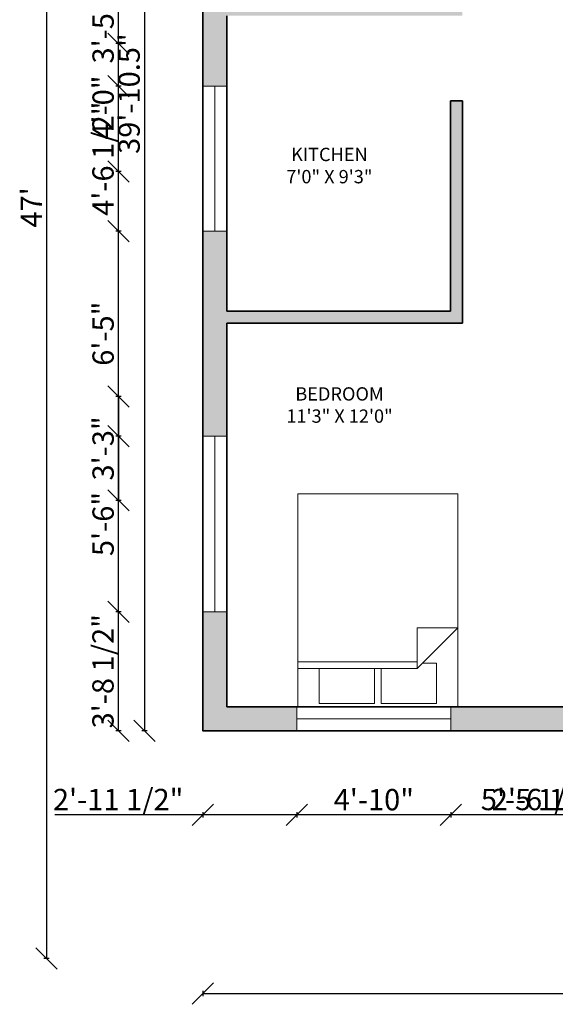
# Model space of a CAD drawing. Units: inches. Extents: x 2561 to 3163, y 493 to 1211.
# Tile 1 of 8: x 2561 to 2762, y 512 to 882. Entities that reach past the tile are written whole.
import ezdxf

# ---------------------------------------------------------------- set-up
doc = ezdxf.new("R2010")
doc.units = ezdxf.units.IN
for name, color, linetype, lineweight in [('A-ANNO-DIMS', 2, 'Continuous', 18), ('A-AREA-IDEN', 7, 'Continuous', 18), ('A-FURN', 8, 'Continuous', 18), ('A-GLAZ', 4, 'Continuous', 18), ('A-WALL', 7, 'Continuous', 35), ('A-WALL-PATT', 24, 'Continuous', 13)]:
    doc.layers.add(name, color=color, linetype=linetype, lineweight=lineweight)
doc.styles.get("Standard").update_dxf_attribs({"font": 'arial.ttf'})
doc.dimstyles.new('ISO-25', dxfattribs={"dimtxt": 8, "dimasz": 8, "dimexe": 1, "dimexo": 1, "dimtad": 1, "dimlunit": 3, "dimtxsty": 'Standard', "dimblk": 'OBLIQUE', "dimcen": 2.5, "dimadec": 0, "dimazin": 0, "dimtfac": 1, "dimtmove": 0, "dimatfit": 3, "dimfxl": 1, "dimfxlon": 1, "dimarcsym": 0})

# ---------------------------------------------------------------- blocks, each defined once
blk = doc.blocks.new('Bed - Queen')
for p, q in [((0, -80.00003), (0, 0)), ((0, 0), (59.99999, 0)), ((59.99999, 0), (59.99999, -80.00003)), ((7.99999, -1.2), (28.79998, -1.2)), ((7.99999, -14.4), (7.99999, -1.2)), ((28.79998, -1.2), (28.79998, -14.4)), ((31.19999, -1.2), (51.99999, -1.2)), ((31.19999, -14.4), (31.19999, -1.2)), ((51.99999, -1.2), (51.99999, -16.4)), ((0, -14.4), (44.8, -14.4)), ((59.99999, -29.6), (44.8, -14.4)), ((44.8, -14.4), (44.8, -29.6)), ((44.8, -16.8), (0, -16.8)), ((51.99999, -16.4), (46.79936, -16.4)), ((44.8, -29.6), (59.99999, -29.6)), ((59.99999, -80.00003), (0, -80.00003))]:
    blk.add_line(p, q)
blk = doc.blocks.new('_Oblique')
at = {"color": 0, "linetype": 'ByBlock', "lineweight": -2}
blk.add_line((-0.5, -0.5), (0.5, 0.5), dxfattribs=at)
blk = doc.blocks.new('*D15')
at = {"layer": 'A-ANNO-DIMS', "color": 0, "lineweight": -2, "transparency": 16777216}
for p, q in [((2629.27, 516.82), (2629.27, 514.82)), ((2629.27, 515.82), (2948.92, 515.82)), ((2948.92, 516.82), (2948.92, 514.82))]:
    blk.add_line(p, q, dxfattribs=at)
at = {"layer": 'Defpoints', "color": 0, "transparency": 16777216}
for p in [(2629.27, 614.57), (2948.92, 614.57), (2948.92, 515.82)]:
    blk.add_point(p, dxfattribs=at)
at = {"layer": 'A-ANNO-DIMS', "color": 0, "lineweight": -2, "transparency": 16777216, "xscale": 8, "yscale": 8, "zscale": 8, "rotation": 180}
blk.add_blockref('_Oblique', (2629.27, 515.82), dxfattribs=at)
at = {"layer": 'A-ANNO-DIMS', "color": 0, "lineweight": -2, "transparency": 16777216, "xscale": 8, "yscale": 8, "zscale": 8}
blk.add_blockref('_Oblique', (2948.92, 515.82), dxfattribs=at)
at = {"layer": 'A-ANNO-DIMS', "color": 0, "transparency": 16777216, "insert": (2789.1, 520.53), "char_height": 8, "attachment_point": 5}
blk.add_mtext('26\'-7.64"', dxfattribs=at)
blk = doc.blocks.new('*D16')
at = {"layer": 'A-ANNO-DIMS', "color": 0, "lineweight": -2, "transparency": 16777216}
for p, q in [((2608.39, 1093.07), (2606.39, 1093.07)), ((2607.39, 1093.07), (2607.39, 614.57)), ((2608.39, 614.57), (2606.39, 614.57))]:
    blk.add_line(p, q, dxfattribs=at)
at = {"layer": 'Defpoints', "color": 0, "transparency": 16777216}
for p in [(2629.27, 1093.07), (2607.39, 614.57), (2629.27, 614.57)]:
    blk.add_point(p, dxfattribs=at)
at = {"layer": 'A-ANNO-DIMS', "color": 0, "lineweight": -2, "transparency": 16777216, "xscale": 8, "yscale": 8, "zscale": 8}
for p, rotation in [((2607.39, 1093.07), 90), ((2607.39, 614.57), 270)]:
    blk.add_blockref('_Oblique', p, dxfattribs=dict(at, rotation=rotation))
at = {"layer": 'A-ANNO-DIMS', "color": 0, "transparency": 16777216, "insert": (2602.67, 853.82), "char_height": 8, "attachment_point": 5, "rotation": 90}
blk.add_mtext('39\'-10.5"', dxfattribs=at)
blk = doc.blocks.new('*D17')
at = {"layer": 'A-ANNO-DIMS', "color": 0, "lineweight": -2, "transparency": 16777216}
for p, q in [((2571.63, 1093.07), (2569.63, 1093.07)), ((2570.63, 1093.07), (2570.63, 529.07)), ((2571.63, 529.07), (2569.63, 529.07))]:
    blk.add_line(p, q, dxfattribs=at)
at = {"layer": 'Defpoints', "color": 0, "transparency": 16777216}
for p in [(2629.27, 1093.07), (2570.63, 529.07), (3109.27, 529.07)]:
    blk.add_point(p, dxfattribs=at)
at = {"layer": 'A-ANNO-DIMS', "color": 0, "lineweight": -2, "transparency": 16777216, "xscale": 8, "yscale": 8, "zscale": 8}
for p, rotation in [((2570.63, 1093.07), 90), ((2570.63, 529.07), 270)]:
    blk.add_blockref('_Oblique', p, dxfattribs=dict(at, rotation=rotation))
at = {"layer": 'A-ANNO-DIMS', "color": 0, "transparency": 16777216, "insert": (2566, 811.07), "char_height": 8, "attachment_point": 5, "rotation": 90}
blk.add_mtext("47'", dxfattribs=at)
blk = doc.blocks.new('*D30')
at = {"layer": 'A-ANNO-DIMS', "color": 0, "lineweight": -2, "transparency": 16777216}
for p, q in [((2598.62, 740.07), (2596.62, 740.07)), ((2597.62, 740.07), (2597.62, 701.07)), ((2598.62, 701.07), (2596.62, 701.07))]:
    blk.add_line(p, q, dxfattribs=at)
at = {"layer": 'Defpoints', "color": 0, "transparency": 16777216}
for p in [(3014.77, 740.07), (2597.62, 701.07), (3014.77, 701.07)]:
    blk.add_point(p, dxfattribs=at)
at = {"layer": 'A-ANNO-DIMS', "color": 0, "lineweight": -2, "transparency": 16777216, "xscale": 8, "yscale": 8, "zscale": 8}
for p, rotation in [((2597.62, 740.07), 90), ((2597.62, 701.07), 270)]:
    blk.add_blockref('_Oblique', p, dxfattribs=dict(at, rotation=rotation))
at = {"layer": 'A-ANNO-DIMS', "color": 0, "transparency": 16777216, "insert": (2592.91, 720.57), "char_height": 8, "attachment_point": 5, "rotation": 90}
blk.add_mtext('3\'-3"', dxfattribs=at)
blk = doc.blocks.new('*D31')
at = {"layer": 'A-ANNO-DIMS', "color": 0, "lineweight": -2, "transparency": 16777216}
for p, q in [((2598.62, 872.57), (2596.62, 872.57)), ((2597.62, 824.57), (2597.62, 872.57)), ((2598.62, 824.57), (2596.62, 824.57))]:
    blk.add_line(p, q, dxfattribs=at)
at = {"layer": 'Defpoints', "color": 0, "transparency": 16777216}
for p in [(2597.62, 872.57), (3011.27, 872.57), (3011.27, 824.57)]:
    blk.add_point(p, dxfattribs=at)
at = {"layer": 'A-ANNO-DIMS', "color": 0, "lineweight": -2, "transparency": 16777216, "xscale": 8, "yscale": 8, "zscale": 8}
for p, rotation in [((2597.62, 872.57), 90), ((2597.62, 824.57), 270)]:
    blk.add_blockref('_Oblique', p, dxfattribs=dict(at, rotation=rotation))
at = {"layer": 'A-ANNO-DIMS', "color": 0, "transparency": 16777216, "insert": (2592.91, 848.57), "char_height": 8, "attachment_point": 5, "rotation": 90}
blk.add_mtext('4\'-0"', dxfattribs=at)
blk = doc.blocks.new('*D46')
at = {"layer": 'A-ANNO-DIMS', "color": 0, "lineweight": -2, "transparency": 16777216}
for p, q in [((2598.62, 897.75), (2596.62, 897.75)), ((2597.62, 856.59), (2597.62, 897.75)), ((2598.62, 856.59), (2596.62, 856.59))]:
    blk.add_line(p, q, dxfattribs=at)
at = {"layer": 'Defpoints', "color": 0, "transparency": 16777216}
for p in [(2597.62, 897.75), (2629.27, 897.75), (2629.27, 856.59)]:
    blk.add_point(p, dxfattribs=at)
at = {"layer": 'A-ANNO-DIMS', "color": 0, "lineweight": -2, "transparency": 16777216, "xscale": 8, "yscale": 8, "zscale": 8}
for p, rotation in [((2597.62, 897.75), 90), ((2597.62, 856.59), 270)]:
    blk.add_blockref('_Oblique', p, dxfattribs=dict(at, rotation=rotation))
at = {"layer": 'A-ANNO-DIMS', "color": 0, "transparency": 16777216, "insert": (2592.91, 877.17), "char_height": 8, "attachment_point": 5, "rotation": 90}
blk.add_mtext('3\'-5"', dxfattribs=at)
blk = doc.blocks.new('*D47')
at = {"layer": 'A-ANNO-DIMS', "color": 0, "lineweight": -2, "transparency": 16777216}
for p, q in [((2598.62, 856.59), (2596.62, 856.59)), ((2597.62, 802.18), (2597.62, 856.59)), ((2598.62, 802.18), (2596.62, 802.18))]:
    blk.add_line(p, q, dxfattribs=at)
at = {"layer": 'Defpoints', "color": 0, "transparency": 16777216}
for p in [(2597.62, 856.59), (2629.27, 856.59), (2629.27, 802.18)]:
    blk.add_point(p, dxfattribs=at)
at = {"layer": 'A-ANNO-DIMS', "color": 0, "lineweight": -2, "transparency": 16777216, "xscale": 8, "yscale": 8, "zscale": 8}
for p, rotation in [((2597.62, 856.59), 90), ((2597.62, 802.18), 270)]:
    blk.add_blockref('_Oblique', p, dxfattribs=dict(at, rotation=rotation))
at = {"layer": 'A-ANNO-DIMS', "color": 0, "transparency": 16777216, "insert": (2592.86, 829.38), "char_height": 8, "attachment_point": 5, "rotation": 90}
blk.add_mtext('4\'-6 1/2"', dxfattribs=at)
blk = doc.blocks.new('*D48')
at = {"layer": 'A-ANNO-DIMS', "color": 0, "lineweight": -2, "transparency": 16777216}
for p, q in [((2598.62, 802.18), (2596.62, 802.18)), ((2597.62, 725.14), (2597.62, 802.18)), ((2598.62, 725.14), (2596.62, 725.14))]:
    blk.add_line(p, q, dxfattribs=at)
at = {"layer": 'Defpoints', "color": 0, "transparency": 16777216}
for p in [(2597.62, 802.18), (2629.27, 802.18), (2629.27, 725.14)]:
    blk.add_point(p, dxfattribs=at)
at = {"layer": 'A-ANNO-DIMS', "color": 0, "lineweight": -2, "transparency": 16777216, "xscale": 8, "yscale": 8, "zscale": 8}
for p, rotation in [((2597.62, 802.18), 90), ((2597.62, 725.14), 270)]:
    blk.add_blockref('_Oblique', p, dxfattribs=dict(at, rotation=rotation))
at = {"layer": 'A-ANNO-DIMS', "color": 0, "transparency": 16777216, "insert": (2592.91, 763.66), "char_height": 8, "attachment_point": 5, "rotation": 90}
blk.add_mtext('6\'-5"', dxfattribs=at)
blk = doc.blocks.new('*D49')
at = {"layer": 'A-ANNO-DIMS', "color": 0, "lineweight": -2, "transparency": 16777216}
for p, q in [((2598.62, 725.14), (2596.62, 725.14)), ((2597.62, 659.23), (2597.62, 725.14)), ((2598.62, 659.23), (2596.62, 659.23))]:
    blk.add_line(p, q, dxfattribs=at)
at = {"layer": 'Defpoints', "color": 0, "transparency": 16777216}
for p in [(2597.62, 725.14), (2629.27, 725.14), (2629.27, 659.23)]:
    blk.add_point(p, dxfattribs=at)
at = {"layer": 'A-ANNO-DIMS', "color": 0, "lineweight": -2, "transparency": 16777216, "xscale": 8, "yscale": 8, "zscale": 8}
for p, rotation in [((2597.62, 725.14), 90), ((2597.62, 659.23), 270)]:
    blk.add_blockref('_Oblique', p, dxfattribs=dict(at, rotation=rotation))
at = {"layer": 'A-ANNO-DIMS', "color": 0, "transparency": 16777216, "insert": (2592.91, 692.19), "char_height": 8, "attachment_point": 5, "rotation": 90}
blk.add_mtext('5\'-6"', dxfattribs=at)
blk = doc.blocks.new('*D50')
at = {"layer": 'A-ANNO-DIMS', "color": 0, "lineweight": -2, "transparency": 16777216}
for p, q in [((2598.62, 659.23), (2596.62, 659.23)), ((2597.62, 614.57), (2597.62, 659.23)), ((2598.62, 614.57), (2596.62, 614.57))]:
    blk.add_line(p, q, dxfattribs=at)
at = {"layer": 'Defpoints', "color": 0, "transparency": 16777216}
for p in [(2597.62, 659.23), (2629.27, 659.23), (2629.27, 614.57)]:
    blk.add_point(p, dxfattribs=at)
at = {"layer": 'A-ANNO-DIMS', "color": 0, "lineweight": -2, "transparency": 16777216, "xscale": 8, "yscale": 8, "zscale": 8}
for p, rotation in [((2597.62, 659.23), 90), ((2597.62, 614.57), 270)]:
    blk.add_blockref('_Oblique', p, dxfattribs=dict(at, rotation=rotation))
at = {"layer": 'A-ANNO-DIMS', "color": 0, "transparency": 16777216, "insert": (2592.86, 636.9), "char_height": 8, "attachment_point": 5, "rotation": 90}
blk.add_mtext('3\'-8 1/2"', dxfattribs=at)
blk = doc.blocks.new('*D58')
at = {"layer": 'A-ANNO-DIMS', "color": 0, "lineweight": -2, "transparency": 16777216}
for p, q in [((2629.27, 582.92), (2573.76, 582.92)), ((2629.27, 583.92), (2629.27, 581.92)), ((2664.61, 582.92), (2629.27, 582.92)), ((2664.61, 583.92), (2664.61, 581.92))]:
    blk.add_line(p, q, dxfattribs=at)
at = {"layer": 'Defpoints', "color": 0, "transparency": 16777216}
for p in [(2629.27, 614.57), (2664.61, 614.57), (2629.27, 582.92)]:
    blk.add_point(p, dxfattribs=at)
at = {"layer": 'A-ANNO-DIMS', "color": 0, "lineweight": -2, "transparency": 16777216, "xscale": 8, "yscale": 8, "zscale": 8, "rotation": 180}
blk.add_blockref('_Oblique', (2629.27, 582.92), dxfattribs=at)
at = {"layer": 'A-ANNO-DIMS', "color": 0, "lineweight": -2, "transparency": 16777216, "xscale": 8, "yscale": 8, "zscale": 8}
blk.add_blockref('_Oblique', (2664.61, 582.92), dxfattribs=at)
at = {"layer": 'A-ANNO-DIMS', "color": 0, "transparency": 16777216, "insert": (2597.52, 587.68), "char_height": 8, "attachment_point": 5}
blk.add_mtext('2\'-11 1/2"', dxfattribs=at)
blk = doc.blocks.new('*D59')
at = {"layer": 'A-ANNO-DIMS', "color": 0, "lineweight": -2, "transparency": 16777216}
for p, q in [((2664.61, 583.92), (2664.61, 581.92)), ((2722.43, 582.92), (2664.61, 582.92)), ((2722.43, 583.92), (2722.43, 581.92))]:
    blk.add_line(p, q, dxfattribs=at)
at = {"layer": 'Defpoints', "color": 0, "transparency": 16777216}
for p in [(2664.61, 614.57), (2722.43, 614.57), (2664.61, 582.92)]:
    blk.add_point(p, dxfattribs=at)
at = {"layer": 'A-ANNO-DIMS', "color": 0, "lineweight": -2, "transparency": 16777216, "xscale": 8, "yscale": 8, "zscale": 8, "rotation": 180}
blk.add_blockref('_Oblique', (2664.61, 582.92), dxfattribs=at)
at = {"layer": 'A-ANNO-DIMS', "color": 0, "lineweight": -2, "transparency": 16777216, "xscale": 8, "yscale": 8, "zscale": 8}
blk.add_blockref('_Oblique', (2722.43, 582.92), dxfattribs=at)
at = {"layer": 'A-ANNO-DIMS', "color": 0, "transparency": 16777216, "insert": (2693.52, 587.63), "char_height": 8, "attachment_point": 5}
blk.add_mtext('4\'-10"', dxfattribs=at)
blk = doc.blocks.new('*D60')
at = {"layer": 'A-ANNO-DIMS', "color": 0, "lineweight": -2, "transparency": 16777216}
for p, q in [((2722.43, 583.92), (2722.43, 581.92)), ((2787.91, 582.92), (2722.43, 582.92)), ((2787.91, 583.92), (2787.91, 581.92))]:
    blk.add_line(p, q, dxfattribs=at)
at = {"layer": 'Defpoints', "color": 0, "transparency": 16777216}
for p in [(2722.43, 614.57), (2787.91, 614.57), (2722.43, 582.92)]:
    blk.add_point(p, dxfattribs=at)
at = {"layer": 'A-ANNO-DIMS', "color": 0, "lineweight": -2, "transparency": 16777216, "xscale": 8, "yscale": 8, "zscale": 8, "rotation": 180}
blk.add_blockref('_Oblique', (2722.43, 582.92), dxfattribs=at)
at = {"layer": 'A-ANNO-DIMS', "color": 0, "lineweight": -2, "transparency": 16777216, "xscale": 8, "yscale": 8, "zscale": 8}
blk.add_blockref('_Oblique', (2787.91, 582.92), dxfattribs=at)
at = {"layer": 'A-ANNO-DIMS', "color": 0, "transparency": 16777216, "insert": (2755.17, 587.68), "char_height": 8, "attachment_point": 5}
blk.add_mtext('5\'-5 1/2"', dxfattribs=at)
blk = doc.blocks.new('*D61')
at = {"layer": 'A-ANNO-DIMS', "color": 0, "lineweight": -2, "transparency": 16777216}
for p, q in [((2787.91, 582.92), (2738.61, 582.92)), ((2787.91, 583.92), (2787.91, 581.92)), ((2818.29, 582.92), (2787.91, 582.92)), ((2818.29, 583.92), (2818.29, 581.92))]:
    blk.add_line(p, q, dxfattribs=at)
at = {"layer": 'Defpoints', "color": 0, "transparency": 16777216}
for p in [(2787.91, 614.57), (2818.29, 614.57), (2787.91, 582.92)]:
    blk.add_point(p, dxfattribs=at)
at = {"layer": 'A-ANNO-DIMS', "color": 0, "lineweight": -2, "transparency": 16777216, "xscale": 8, "yscale": 8, "zscale": 8, "rotation": 180}
blk.add_blockref('_Oblique', (2787.91, 582.92), dxfattribs=at)
at = {"layer": 'A-ANNO-DIMS', "color": 0, "lineweight": -2, "transparency": 16777216, "xscale": 8, "yscale": 8, "zscale": 8}
blk.add_blockref('_Oblique', (2818.29, 582.92), dxfattribs=at)
at = {"layer": 'A-ANNO-DIMS', "color": 0, "transparency": 16777216, "insert": (2759.26, 587.68), "char_height": 8, "attachment_point": 5}
blk.add_mtext('2\'-6 1/2"', dxfattribs=at)

msp = doc.modelspace()

# ---------------------------------------------------------------- hatches: boundary and pattern name
at = {"layer": 'A-WALL-PATT'}
h = msp.add_hatch(color=256, dxfattribs=at)
h.dxf.hatch_style = 1
h.paths.add_polyline_path([(2665.022, 1093.069), (2629.274, 1093.069), (2629.274, 1056.034), (2638.274, 1056.034), (2638.274, 1084.069), (2665.022, 1084.069)])
h.paths.add_polyline_path([(2785.37, 1093.069), (2727.193, 1093.069), (2727.193, 1084.069), (2773.274, 1084.069), (2773.274, 940.069), (2762.774, 940.069), (2762.774, 935.569), (2777.774, 935.569), (2777.774, 971.569), (2825.774, 971.569), (2825.774, 935.569), (2921.774, 935.569), (2921.774, 940.069), (2830.274, 940.069), (2830.274, 976.069), (2777.774, 976.069), (2777.774, 1084.069), (2785.37, 1084.069)])
h.paths.add_polyline_path([(2856.568, 1093.069), (2816.168, 1093.069), (2816.168, 1084.069), (2825.774, 1084.069), (2825.774, 1008.069), (2830.274, 1008.069), (2830.274, 1084.069), (2856.568, 1084.069)], flags=17)
h.paths.add_polyline_path([(3006.866, 1093.069), (2929.24, 1093.069), (2929.24, 1084.069), (2962.274, 1084.069), (2962.274, 940.069), (2957.774, 940.069), (2957.774, 935.569), (2970.774, 935.569), (2970.774, 940.069), (2968.274, 940.069), (2968.274, 1084.069), (3006.866, 1084.069)])
h.paths.add_polyline_path([(3109.274, 1093.069), (3068.804, 1093.069), (3068.804, 1084.069), (3100.274, 1084.069), (3100.274, 1061.194), (3109.274, 1061.194)])
h.paths.add_polyline_path([(3109.274, 991.723), (3100.274, 991.723), (3100.274, 940.069), (3010.774, 940.069), (3010.774, 935.569), (3010.774, 911.569), (3015.274, 911.569), (3015.274, 935.569), (3100.274, 935.569), (3100.274, 927.07), (3109.274, 927.07)])
h.paths.add_polyline_path([(3109.274, 897.327), (3100.274, 897.327), (3100.274, 881.569), (2957.774, 881.569), (2957.774, 872.569), (3100.274, 872.569), (3100.274, 805.791), (3109.274, 805.791)])
h.paths.add_polyline_path([(2638.274, 982.372), (2629.274, 982.372), (2629.274, 927.027), (2638.274, 927.027), (2638.274, 935.569), (2722.274, 935.569), (2722.274, 919.569), (2726.774, 919.569), (2726.774, 940.069), (2638.274, 940.069)])
h.paths.add_polyline_path([(2638.274, 883.069), (2726.774, 883.069), (2726.774, 887.569), (2638.274, 887.569), (2638.274, 897.75), (2629.274, 897.75), (2629.274, 856.591), (2638.274, 856.591)])
h.paths.add_polyline_path([(2726.774, 851.069), (2722.274, 851.069), (2722.274, 772.069), (2638.274, 772.069), (2638.274, 802.178), (2629.274, 802.178), (2629.274, 725.136), (2638.274, 725.136), (2638.274, 767.569), (2726.774, 767.569)])
h.paths.add_polyline_path([(2638.274, 659.235), (2629.274, 659.235), (2629.274, 614.569), (2638.274, 614.569)])
h.paths.add_polyline_path([(2664.613, 623.569), (2638.274, 623.569), (2638.274, 614.569), (2664.613, 614.569)])
h.paths.add_polyline_path([(2787.908, 623.569), (2777.774, 623.569), (2777.774, 767.569), (2825.774, 767.569), (2825.774, 659.569), (2830.274, 659.569), (2830.274, 767.569), (2836.774, 767.569), (2836.774, 772.069), (2766.674, 772.069), (2766.674, 767.569), (2773.274, 767.569), (2773.274, 623.569), (2722.435, 623.569), (2722.435, 614.569), (2787.908, 614.569)])
h.paths.add_polyline_path([(2883.664, 623.569), (2867.474, 623.569), (2818.294, 623.569), (2818.294, 614.569), (2883.664, 614.569)])
h.paths.add_polyline_path([(2965.274, 772.069), (2872.774, 772.069), (2872.774, 767.569), (2962.274, 767.569), (2962.274, 623.569), (2936.565, 623.569), (2936.565, 614.569), (2965.274, 614.569)])
h.paths.add_polyline_path([(3109.274, 758.846), (3100.274, 758.846), (3100.274, 701.069), (3013.274, 701.069), (3013.274, 695.069), (3109.274, 695.069)])
h.paths.add_polyline_path([(2965.274, 824.569), (2957.774, 824.569), (2957.774, 772.069), (2965.274, 772.069)])

# ---------------------------------------------------------------- linework, layer by layer
at = {"layer": 'A-GLAZ'}
for p, q in [((2638.274, 856.591), (2629.274, 856.591)), ((2638.274, 802.178), (2629.274, 802.178)), ((2638.274, 725.136), (2629.274, 725.136)), ((2638.274, 659.235), (2629.274, 659.235)), ((2664.613, 623.569), (2664.613, 614.569)), ((2722.435, 623.569), (2722.435, 614.569)), ((2664.613, 619.069), (2722.435, 619.069))]:
    msp.add_line(p, q, dxfattribs=at)
for points in [[(2633.774, 856.591), (2633.774, 802.178)], [(2633.774, 725.136), (2633.774, 659.235)]]:
    msp.add_lwpolyline(points, dxfattribs=at)
at = {"layer": 'A-WALL'}
for p, q in [((2638.274, 883.069), (2638.274, 772.069)), ((2722.274, 851.069), (2722.274, 772.069)), ((2722.274, 851.069), (2726.774, 851.069)), ((2726.774, 767.569), (2726.774, 851.069)), ((2722.274, 772.069), (2638.274, 772.069)), ((2726.774, 767.569), (2638.274, 767.569)), ((2638.274, 767.569), (2638.274, 623.569)), ((2773.274, 623.569), (2638.274, 623.569))]:
    msp.add_line(p, q, dxfattribs=at)
msp.add_lwpolyline([(3109.274, 695.069), (3109.274, 1093.069), (2629.274, 1093.069), (2629.274, 614.569), (2965.274, 614.569)], dxfattribs=at)

# ---------------------------------------------------------------- block references
at = {"layer": 'A-FURN', "xscale": -1, "rotation": 180}
msp.add_blockref('Bed - Queen', (2665.022, 623.569), dxfattribs=at)

# ---------------------------------------------------------------- texts
at = {"layer": 'A-AREA-IDEN', "char_height": 5, "attachment_point": 1}
for s, insert in [('\\pxqc;KITCHEN\\P7\'0" X 9\'3"', (2646.206, 833.461)), ('\\pxqc;BEDROOM\\P11\'3" X 12\'0"', (2650.014, 743.539))]:
    msp.add_mtext_dynamic_manual_height_columns(s, width=61.24894, gutter_width=12.5, heights=[0], dxfattribs=dict(at, insert=insert))

# ---------------------------------------------------------------- dimensions: what is measured, and where the dimension line sits
at = {"layer": 'A-ANNO-DIMS'}
for base, p1, p2, angle, override, picture, middle in [((2570.627, 529.069), (2629.274, 1093.069), (3109.274, 529.069), 90, {"dimclrd": 0, "dimclre": 0, "dimclrt": 0}, '*D17', (2566.002, 811.069)), ((2607.386, 614.569), (2629.274, 1093.069), (2629.274, 614.569), 90, {"dimclrd": 0, "dimclre": 0, "dimclrt": 0}, '*D16', (2602.674, 853.819)), ((2597.624, 897.75), (2629.274, 856.591), (2629.274, 897.75), 90, {"dimdec": 1, "dimlfac": 1, "dimrnd": 0, "dimzin": 1, "dimdsep": 46, "dimlunit": 4, "dimfrac": 2}, '*D46', (2592.911, 877.171)), ((2597.624, 872.569), (3011.274, 824.569), (3011.274, 872.569), 90, {"dimdec": 1, "dimlfac": 1, "dimrnd": 0, "dimzin": 1, "dimdsep": 46, "dimlunit": 4, "dimfrac": 2}, '*D31', (2592.914, 848.569)), ((2597.624, 856.591), (2629.274, 802.178), (2629.274, 856.591), 90, {"dimdec": 1, "dimlfac": 1, "dimrnd": 0, "dimzin": 1, "dimdsep": 46, "dimlunit": 4, "dimfrac": 2}, '*D47', (2592.862, 829.385)), ((2597.624, 802.178), (2629.274, 725.136), (2629.274, 802.178), 90, {"dimdec": 1, "dimlfac": 1, "dimrnd": 0, "dimzin": 1, "dimdsep": 46, "dimlunit": 4, "dimfrac": 2}, '*D48', (2592.914, 763.657)), ((2597.624, 701.069), (3014.774, 740.069), (3014.774, 701.069), 90, {"dimdec": 1, "dimlfac": 1, "dimrnd": 0, "dimzin": 1, "dimdsep": 46, "dimlunit": 4, "dimfrac": 2}, '*D30', (2592.911, 720.569)), ((2597.624, 725.136), (2629.274, 659.235), (2629.274, 725.136), 90, {"dimdec": 1, "dimlfac": 1, "dimrnd": 0, "dimzin": 1, "dimdsep": 46, "dimlunit": 4, "dimfrac": 2}, '*D49', (2592.914, 692.185)), ((2597.624, 659.235), (2629.274, 614.569), (2629.274, 659.235), 90, {"dimdec": 1, "dimlfac": 1, "dimrnd": 0, "dimzin": 1, "dimdsep": 46, "dimlunit": 4, "dimfrac": 2}, '*D50', (2592.86, 636.902)), ((2629.274, 582.919), (2664.613, 614.569), (2629.274, 614.569), 180, {"dimdec": 1, "dimlfac": 1, "dimrnd": 0, "dimzin": 1, "dimdsep": 46, "dimlunit": 4, "dimfrac": 2}, '*D58', (2597.519, 587.68)), ((2664.613, 582.919), (2722.435, 614.569), (2664.613, 614.569), 180, {"dimdec": 1, "dimlfac": 1, "dimrnd": 0, "dimzin": 1, "dimdsep": 46, "dimlunit": 4, "dimfrac": 2}, '*D59', (2693.524, 587.628)), ((2722.435, 582.919), (2787.908, 614.569), (2722.435, 614.569), 180, {"dimdec": 1, "dimlfac": 1, "dimrnd": 0, "dimzin": 1, "dimdsep": 46, "dimlunit": 4, "dimfrac": 2}, '*D60', (2755.171, 587.68)), ((2787.908, 582.919), (2818.294, 614.569), (2787.908, 614.569), 180, {"dimdec": 1, "dimlfac": 1, "dimrnd": 0, "dimzin": 1, "dimdsep": 46, "dimlunit": 4, "dimfrac": 2}, '*D61', (2759.261, 587.68))]:
    dim = msp.add_linear_dim(base=base, p1=p1, p2=p2, angle=angle, dimstyle='ISO-25', override=override, dxfattribs=at)
    dim.commit()
    dim.dimension.update_dxf_attribs({"geometry": picture, "text_midpoint": middle})
dim = msp.add_linear_dim(base=(2948.918, 515.818), p1=(2629.274, 614.569), p2=(2948.918, 614.569), dimstyle='ISO-25', override={"dimclrd": 0, "dimclre": 0, "dimclrt": 0}, dxfattribs=at)
dim.commit()
dim.dimension.update_dxf_attribs({"geometry": '*D15', "text_midpoint": (2789.096, 520.527)})

doc.saveas('drawing.dxf')
